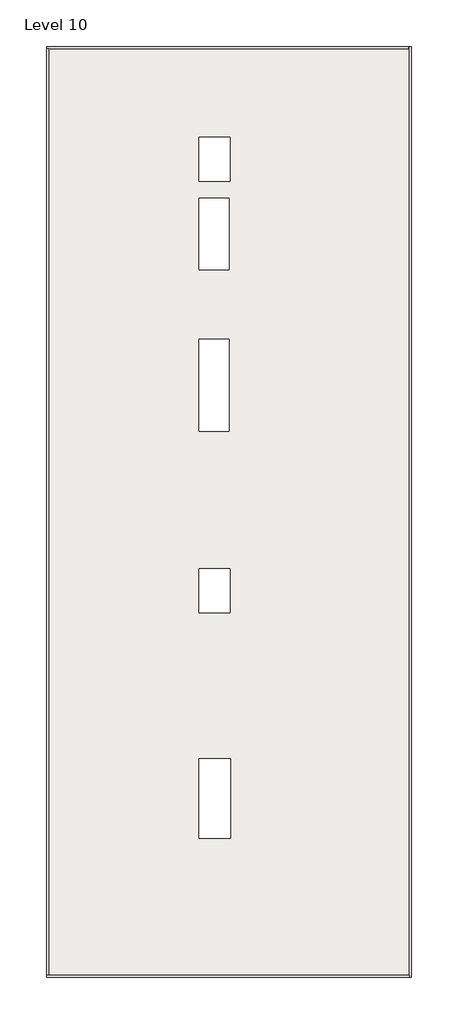
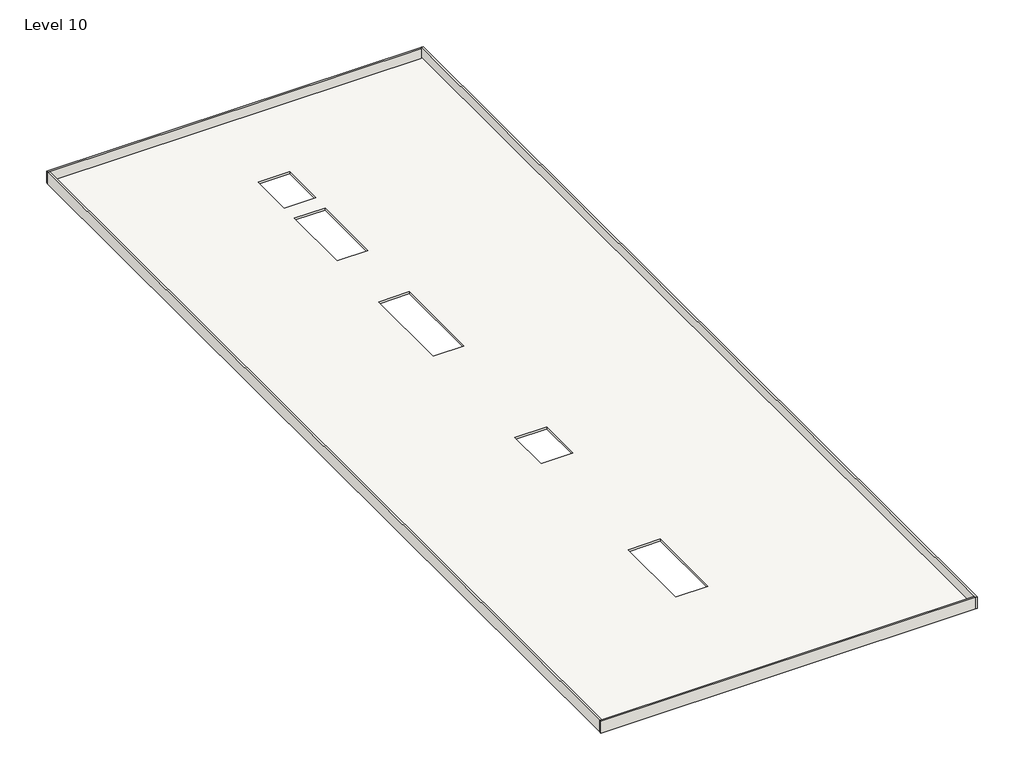
# One storey: 4 walls, 1 roof.
"""IFC4 building model written with IfcOpenShell, lengths in millimetres."""

from ifc_helpers import new_model, si_unit, frame, origin, place, context, project, spatial, polyline, outline, extrude, faceted_brep, element, save

model = new_model("IFC4")

# Units and contexts
model_context = context("Model", 3, world=origin())
ifc_project = project(units=[si_unit("LENGTHUNIT", "METRE", prefix="MILLI")], contexts=[model_context])

# Site, building, storey
site = spatial("IfcSite", under=ifc_project)
building = spatial("IfcBuilding", under=site)
storey = spatial("IfcBuildingStorey", under=building, Name="Level 10", Elevation=52666.6172466)

# Roof
placement = place(None, origin())
element("IfcRoof", 1, ObjectType="SLAB", at=placement, inside=storey, context=model_context, shape_type="SweptSolid", body=[
    extrude(outline(polyline([(-15237.9415084, -35021.5344126), (-15237.9415084, 36097.9216096), (12498.9443719, 36097.9216096), (12498.9443719, -35021.5344126), (-15237.9415084, -35021.5344126)]), holes=[polyline([(-3617.4415084, 29152.4900967), (-3617.4415084, 25799.6900967), (-1255.2415084, 25799.6900967), (-1255.2415084, 29152.4900967), (-3617.4415084, 29152.4900967)]), polyline([(-3617.4415084, 24490.1216096), (-3617.4415084, 19003.7216096), (-1331.4415084, 19003.7216096), (-1331.4415084, 24490.1216096), (-3617.4415084, 24490.1216096)]), polyline([(-3617.4415084, 13669.6303368), (-3617.4415084, 6659.2303368), (-1331.4415084, 6659.2303368), (-1331.4415084, 13669.6303368), (-3617.4415084, 13669.6303368)]), polyline([(-3617.4415084, -3882.2751812), (-3617.4415084, -7235.0751812), (-1255.2415084, -7235.0751812), (-1255.2415084, -3882.2751812), (-3617.4415084, -3882.2751812)]), polyline([(-3617.4415084, -18429.9851539), (-3617.4415084, -24525.9851539), (-1229.8415084, -24525.9851539), (-1229.8415084, -18429.9851539), (-3617.4415084, -18429.9851539)])]), frame((0.0, 0.0, 52666.6172466), z_axis=(0.0, 0.0, 1.0), x_axis=(1.0, 0.0, 0.0)), (0.0, 0.0, 1.0), 152.4),
])

# Walls
element("IfcWall", 2, ObjectType="6\"", at=placement, inside=storey, context=model_context, shape_type="Brep", body=[
    faceted_brep([(-15314.1415084, 35945.5216096, 52666.6172466), (-15161.7415084, 35945.5216096, 52666.6172466), (12422.7443719, 35945.5216096, 52666.6172466), (12422.7443719, 35945.5216096, 53581.0172466), (-15161.7415084, 35945.5216096, 53581.0172466), (-15314.1415084, 35945.5216096, 53581.0172466), (-15314.1415084, 36097.9216096, 52666.6172466), (-15314.1415084, 36097.9216096, 53581.0172466), (12422.7443719, 36097.9216096, 53581.0172466), (12422.7443719, 36097.9216096, 52666.6172466)], [[[0, 1, 2, 3, 4, 5]], [[6, 7, 8, 9]], [[2, 1, 0, 6, 9]], [[3, 2, 9, 8]], [[5, 4, 3, 8, 7]], [[0, 5, 7, 6]]]),
])
element("IfcWall", 3, ObjectType="6\"", at=placement, inside=storey, context=model_context, shape_type="Brep", body=[
    faceted_brep([(12498.9443719, 36097.9216096, 52666.6172466), (12498.9443719, -35021.5344126, 52666.6172466), (12498.9443719, -35173.9344126, 52666.6172466), (12498.9443719, -35173.9344126, 53581.0172466), (12498.9443719, -35021.5344126, 53581.0172466), (12498.9443719, 36097.9216096, 53581.0172466), (12651.3443719, 36097.9216096, 52666.6172466), (12651.3443719, 36097.9216096, 53581.0172466), (12651.3443719, -35173.9344126, 53581.0172466), (12651.3443719, -35173.9344126, 52666.6172466)], [[[0, 1, 2, 3, 4, 5]], [[6, 7, 8, 9]], [[2, 1, 0, 6, 9]], [[5, 4, 3, 8, 7]], [[0, 5, 7, 6]], [[3, 2, 9, 8]]]),
])
element("IfcWall", 4, ObjectType="6\"", at=placement, inside=storey, context=model_context, shape_type="Brep", body=[
    faceted_brep([(12498.9443719, -35021.5344126, 52666.6172466), (-15161.7415084, -35021.5344126, 52666.6172466), (-15314.1415084, -35021.5344126, 52666.6172466), (-15314.1415084, -35021.5344126, 53581.0172466), (-15161.7415084, -35021.5344126, 53581.0172466), (12498.9443719, -35021.5344126, 53581.0172466), (12498.9443719, -35173.9344126, 52666.6172466), (12498.9443719, -35173.9344126, 53581.0172466), (-15314.1415084, -35173.9344126, 53581.0172466), (-15314.1415084, -35173.9344126, 52666.6172466)], [[[0, 1, 2, 3, 4, 5]], [[6, 7, 8, 9]], [[2, 1, 0, 6, 9]], [[5, 4, 3, 8, 7]], [[0, 5, 7, 6]], [[3, 2, 9, 8]]]),
])
element("IfcWall", 5, ObjectType="6\"", at=placement, inside=storey, context=model_context, shape_type="SweptSolid", body=[
    extrude(outline(polyline([(-15161.7415084, 35945.5216096), (-15161.7415084, -35021.5344126), (-15314.1415084, -35021.5344126), (-15314.1415084, 35945.5216096), (-15161.7415084, 35945.5216096)])), frame((0.0, 0.0, 52666.6172466), z_axis=(0.0, 0.0, 1.0), x_axis=(1.0, 0.0, 0.0)), (0.0, 0.0, 1.0), 914.4),
])

save(model, "model.ifc")

# Revit data of these elements
# Type "SLAB"
#   Assembly Code = "B1020"
#   Layers, outside or top first: 0' - 6" "Damp-proofing" (function 1)
# Type "6\""
#   Assembly Code = "B2010"
#   Layers, outside or top first: 0' - 6" "WALLS" (function 1)
# Element 1 (IfcRoof, "SLAB")
#   built-in parameter 1001705 = 173.291 (stored number, unit not read)
#   built-in parameter 1001710 = 33615
#   Phase Created = New Construction
#   Materials on its faces: "Damp-proofing"
# Elements 2, 3, 4, 5 (IfcWall, "6\"")
#   Top Offset = 0' - 0"
#   Base Offset = 0' - 0"
#   Unconnected Height = 3' - 0"
#   wall height = 3' - 0"
#   Phase Created = New Construction
#   Base Constraint = Level 10
#   Materials on its faces: "WALLS"
# Materials
#   "Damp-proofing": class "Generic", colour RGB 127 127 127, transparency 0, Description = "Damp-proofing", Cost = 0
#   "WALLS": class "Generic", colour RGB 120 120 120, transparency 0, Cost = 0
